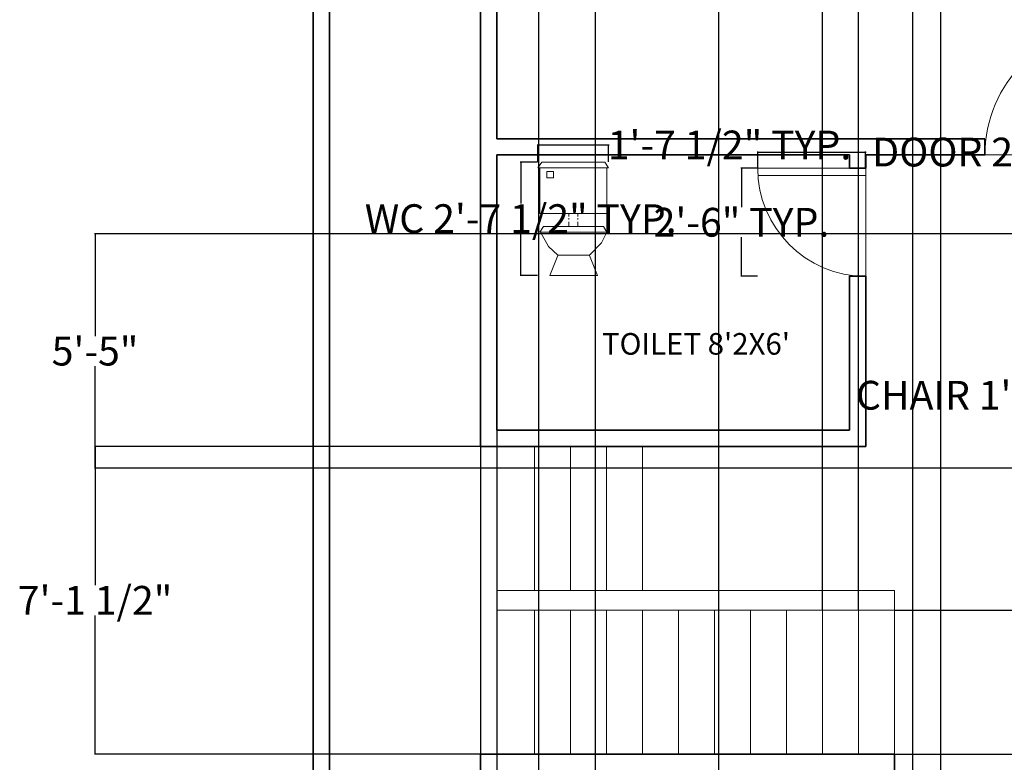
# Model space of a CAD drawing. Units: inches. Extents: x -438 to 102, y -60 to 1091.
# Tile 4 of 20: x -436 to -162, y 492 to 699. Entities that reach past the tile are written whole.
import ezdxf

# ---------------------------------------------------------------- set-up
doc = ezdxf.new("R2010")
doc.units = ezdxf.units.IN
doc.header["$MEASUREMENT"] = 0
for name, color, linetype, lineweight, true_color in [('A-ANNO-DIMS', 217, 'Continuous', 18, 0x93278f), ('A-DOOR', 30, 'Continuous', 18, 0xf26722), ('A-WALL', 2, 'Continuous', 35, 0xf1eb1f), ('C-PROP', 2, 'Continuous', 35, 0xf1eb1f)]:
    doc.layers.add(name, color=color, linetype=linetype, lineweight=lineweight, true_color=true_color)
for name, color, linetype, lineweight in [('A-AREA-IDEN', 4, 'Continuous', 18), ('A-FLOR-FIXT', 9, 'Continuous', 15), ('A-FLOR-STRS', 7, 'Continuous', 18)]:
    doc.layers.add(name, color=color, linetype=linetype, lineweight=lineweight)
doc.styles.get("Standard").update_dxf_attribs({"font": 'arial.ttf'})
doc.dimstyles.get("Standard").update_dxf_attribs({"dimtxt": 8, "dimasz": 0.18, "dimexe": 0.18, "dimexo": 0.0625, "dimgap": 0.09, "dimtad": 0, "dimtih": 1, "dimtoh": 1, "dimdec": 4, "dimzin": 0, "dimdsep": 46, "dimlunit": 3, "dimtxsty": 'Standard', "dimcen": 0.09, "dimadec": 0, "dimazin": 0, "dimtfac": 1, "dimtdec": 4, "dimtofl": 0, "dimtmove": 0, "dimatfit": 3, "dimfxl": 1, "dimtolj": 1, "dimtzin": 0, "dimarcsym": 0})

# ---------------------------------------------------------------- blocks, each defined once
blk = doc.blocks.new('WC-CLOSE-COUPLED')
for p, q in [((-9.84, -1.66, -13.5), (-8.74, 0, -13.5)), ((-8.74, 0, -13.5), (8.78, 0, -13.5)), ((9.84, -1.66, -13.5), (8.78, 0, -13.5)), ((-9.84, -1.66, -13.5), (9.84, -1.66, -13.5)), ((-9.27, -1.66, -13.5), (-9.27, -14.26, -13.5)), ((-7.35, -2.62, -13.5), (-7.35, -4.39, -13.5)), ((-5.45, -2.62, -13.5), (-7.35, -2.62, -13.5)), ((-5.45, -4.39, -13.5), (-5.45, -2.62, -13.5)), ((9.31, -14.26, -13.5), (9.31, -1.66, -13.5)), ((-7.35, -4.39, -13.5), (-5.45, -4.39, -13.5)), ((-9.27, -14.26, -13.5), (9.31, -14.26, -13.5)), ((-1.22, -15.15, -13.5), (-1.22, -14.23, -13.5)), ((-1.22, -15.97, -13.5), (-1.22, -15.56, -13.5)), ((0.02, -14.26, -13.5), (1.26, -14.26, -13.5)), ((1.26, -14.26, -13.5), (1.26, -15.15, -13.5)), ((1.26, -15.56, -13.5), (1.26, -15.97, -13.5)), ((-9.27, -19.49, -13.5), (-8.25, -17.89, -13.5)), ((-8.25, -17.89, -13.5), (8.4, -17.89, -13.5)), ((-1.22, -17.96, -13.5), (-1.22, -16.65, -13.5)), ((1.26, -17.96, -13.5), (-1.22, -17.96, -13.5)), ((1.26, -16.65, -13.5), (1.26, -17.96, -13.5)), ((9.31, -19.49, -13.5), (8.4, -17.89, -13.5)), ((-9.27, -19.49, -13.5), (9.31, -19.49, -13.5)), ((9.52, -19.49, -13.5), (-9.07, -19.49, -13.5)), ((-9.07, -19.49, -13.5), (-6.87, -23.48, -13.5)), ((7.85, -22.5, -13.5), (9.31, -19.49, -13.5)), ((-6.87, -23.48, -13.5), (-4.26, -25.89, -13.5)), ((4.51, -25.89, -13.5), (7.85, -22.5, -13.5)), ((-6.51, -31.49, -13.5), (-4.3, -25.95, -13.5)), ((-4.26, -25.89, -13.5), (4.51, -25.89, -13.5)), ((4.51, -25.89, -13.5), (-4.26, -25.89, -13.5)), ((6.76, -31.49, -13.5), (4.55, -25.95, -13.5)), ((-6.51, -31.49, -13.5), (6.76, -31.49, -13.5)), ((0.12, -31.49, -13.5), (-6.51, -31.49, -13.5))]:
    blk.add_line(p, q)
blk = doc.blocks.new('DOOR-SWING-36')
for p, q in [((-36, 0), (0, 0)), ((-2, 0), (-2, -36)), ((0, 0), (0, -36))]:
    blk.add_line(p, q)
blk.add_arc((0, 0), 36, 180, 270)
blk = doc.blocks.new('DOOR-SWING-30')
for p, q in [((0, 0), (-30, 0)), ((0, -30), (0, 0)), ((0, -2), (-30, -2))]:
    blk.add_line(p, q)
blk.add_arc((0, 0), 30, 180, 270)
blk = doc.blocks.new('*D14')
at = {"layer": 'A-ANNO-DIMS', "color": 0, "lineweight": -2, "transparency": 16777216}
for p, q in [((-99.6, 597.28), (-99.6, 594.06)), ((-78.92, 597.28), (-78.92, 594.06)), ((-99.6, 594.24), (-99.78, 594.24)), ((-79.1, 594.24), (-99.42, 594.24))]:
    blk.add_line(p, q, dxfattribs=at)
at = {"layer": 'A-ANNO-DIMS', "color": 0, "transparency": 16777216}
for points in [[(-99.42, 594.27), (-99.42, 594.21), (-99.6, 594.24)], [(-79.1, 594.27), (-79.1, 594.21), (-78.92, 594.24)]]:
    blk.add_solid(points, dxfattribs=at)
at = {"layer": 'Defpoints', "color": 0, "transparency": 16777216}
for p in [(-99.6, 597.34), (-78.92, 597.34), (-99.6, 594.24)]:
    blk.add_point(p, dxfattribs=at)
at = {"layer": 'A-ANNO-DIMS', "color": 0, "transparency": 16777216, "insert": (-152.46, 594.24), "char_height": 8, "attachment_point": 5}
blk.add_mtext('\\A1;CHAIR 1\'-8 1/2" TYP.', dxfattribs=at)
blk = doc.blocks.new('*D18')
at = {"layer": 'A-ANNO-DIMS', "color": 0, "lineweight": -2, "transparency": 16777216}
for p, q in [((-291.82, 659.04), (-296.67, 659.04)), ((-296.49, 658.86), (-296.49, 647.52)), ((-296.49, 627.73), (-296.49, 639.07)), ((-291.82, 627.55), (-296.67, 627.55))]:
    blk.add_line(p, q, dxfattribs=at)
at = {"layer": 'A-ANNO-DIMS', "color": 0, "transparency": 16777216}
for points in [[(-296.52, 658.86), (-296.46, 658.86), (-296.49, 659.04)], [(-296.52, 627.73), (-296.46, 627.73), (-296.49, 627.55)]]:
    blk.add_solid(points, dxfattribs=at)
at = {"layer": 'Defpoints', "color": 0, "transparency": 16777216}
for p in [(-296.49, 659.04), (-291.76, 659.04), (-291.76, 627.55)]:
    blk.add_point(p, dxfattribs=at)
at = {"layer": 'A-ANNO-DIMS', "color": 0, "transparency": 16777216, "insert": (-296.49, 643.3), "char_height": 8, "attachment_point": 5}
blk.add_mtext('\\A1;WC 2\'-7 1/2" TYP.', dxfattribs=at)
blk = doc.blocks.new('*D19')
at = {"layer": 'A-ANNO-DIMS', "color": 0, "lineweight": -2, "transparency": 16777216}
for p, q in [((-291.76, 659.11), (-291.76, 663.95)), ((-291.58, 663.77), (-272.26, 663.77)), ((-272.08, 659.11), (-272.08, 663.95)), ((-272.08, 663.77), (-271.9, 663.77))]:
    blk.add_line(p, q, dxfattribs=at)
at = {"layer": 'A-ANNO-DIMS', "color": 0, "transparency": 16777216}
for points in [[(-291.58, 663.8), (-291.58, 663.74), (-291.76, 663.77)], [(-272.26, 663.8), (-272.26, 663.74), (-272.08, 663.77)]]:
    blk.add_solid(points, dxfattribs=at)
at = {"layer": 'Defpoints', "color": 0, "transparency": 16777216}
for p in [(-272.08, 663.77), (-291.76, 659.04), (-272.08, 659.04)]:
    blk.add_point(p, dxfattribs=at)
at = {"layer": 'A-ANNO-DIMS', "color": 0, "transparency": 16777216, "insert": (-238.48, 663.77), "char_height": 8, "attachment_point": 5}
blk.add_mtext('\\A1;1\'-7 1/2" TYP.', dxfattribs=at)
blk = doc.blocks.new('*D22')
at = {"layer": 'A-ANNO-DIMS', "color": 0, "lineweight": -2, "transparency": 16777216}
for p, q in [((-230.65, 657.36), (-230.65, 661.98)), ((-230.47, 661.8), (-200.83, 661.8)), ((-200.65, 657.36), (-200.65, 661.98)), ((-200.65, 661.8), (-200.47, 661.8))]:
    blk.add_line(p, q, dxfattribs=at)
at = {"layer": 'A-ANNO-DIMS', "color": 0, "transparency": 16777216}
for points in [[(-230.47, 661.83), (-230.47, 661.77), (-230.65, 661.8)], [(-200.83, 661.83), (-200.83, 661.77), (-200.65, 661.8)]]:
    blk.add_solid(points, dxfattribs=at)
at = {"layer": 'Defpoints', "color": 0, "transparency": 16777216}
for p in [(-200.65, 661.8), (-230.65, 657.3), (-200.65, 657.3)]:
    blk.add_point(p, dxfattribs=at)
at = {"layer": 'A-ANNO-DIMS', "color": 0, "transparency": 16777216, "insert": (-157.88, 661.8), "char_height": 8, "attachment_point": 5}
blk.add_mtext('\\A1;DOOR 2\'-6" TYP.', dxfattribs=at)
blk = doc.blocks.new('*D23')
at = {"layer": 'A-ANNO-DIMS', "color": 0, "lineweight": -2, "transparency": 16777216}
for p, q in [((-230.71, 657.3), (-235.33, 657.3)), ((-235.15, 657.12), (-235.15, 646.47)), ((-235.15, 627.48), (-235.15, 638.13)), ((-230.71, 627.3), (-235.33, 627.3))]:
    blk.add_line(p, q, dxfattribs=at)
at = {"layer": 'A-ANNO-DIMS', "color": 0, "transparency": 16777216}
for points in [[(-235.18, 657.12), (-235.12, 657.12), (-235.15, 657.3)], [(-235.18, 627.48), (-235.12, 627.48), (-235.15, 627.3)]]:
    blk.add_solid(points, dxfattribs=at)
at = {"layer": 'Defpoints', "color": 0, "transparency": 16777216}
for p in [(-235.15, 657.3), (-230.65, 657.3), (-230.65, 627.3)]:
    blk.add_point(p, dxfattribs=at)
at = {"layer": 'A-ANNO-DIMS', "color": 0, "transparency": 16777216, "insert": (-235.15, 642.3), "char_height": 8, "attachment_point": 5}
blk.add_mtext('\\A1;2\'-6" TYP.', dxfattribs=at)
blk = doc.blocks.new('*D29')
at = {"layer": 'A-ANNO-DIMS', "color": 0, "lineweight": -2, "transparency": 16777216}
for p, q in [((-303.15, 494.44), (-303.15, -48.58)), ((-192.65, 494.44), (-192.65, -48.58)), ((-302.97, -48.4), (-267.94, -48.4)), ((-192.83, -48.4), (-227.85, -48.4))]:
    blk.add_line(p, q, dxfattribs=at)
at = {"layer": 'A-ANNO-DIMS', "color": 0, "transparency": 16777216}
for points in [[(-302.97, -48.37), (-302.97, -48.43), (-303.15, -48.4)], [(-192.83, -48.37), (-192.83, -48.43), (-192.65, -48.4)]]:
    blk.add_solid(points, dxfattribs=at)
at = {"layer": 'Defpoints', "color": 0, "transparency": 16777216}
for p in [(-303.15, 494.5), (-192.65, 494.5), (-192.65, -48.4)]:
    blk.add_point(p, dxfattribs=at)
at = {"layer": 'A-ANNO-DIMS', "color": 0, "transparency": 16777216, "insert": (-247.9, -48.4), "char_height": 8, "attachment_point": 5}
blk.add_mtext('\\A1;9\'-2 1/2"', dxfattribs=at)
blk = doc.blocks.new('*D30')
at = {"layer": 'A-ANNO-DIMS', "color": 0, "lineweight": -2, "transparency": 16777216}
for p, q in [((-303.21, 580), (-414.94, 580)), ((-414.76, 579.82), (-414.76, 541.48)), ((-414.76, 494.68), (-414.76, 533.02)), ((-303.21, 494.5), (-414.94, 494.5))]:
    blk.add_line(p, q, dxfattribs=at)
at = {"layer": 'A-ANNO-DIMS', "color": 0, "transparency": 16777216}
for points in [[(-414.79, 579.82), (-414.73, 579.82), (-414.76, 580)], [(-414.79, 494.68), (-414.73, 494.68), (-414.76, 494.5)]]:
    blk.add_solid(points, dxfattribs=at)
at = {"layer": 'Defpoints', "color": 0, "transparency": 16777216}
for p in [(-414.76, 580), (-303.15, 580), (-303.15, 494.5)]:
    blk.add_point(p, dxfattribs=at)
at = {"layer": 'A-ANNO-DIMS', "color": 0, "transparency": 16777216, "insert": (-414.76, 537.25), "char_height": 8, "attachment_point": 5}
blk.add_mtext('\\A1;7\'-1 1/2"', dxfattribs=at)
blk = doc.blocks.new('*D32')
at = {"layer": 'A-ANNO-DIMS', "color": 0, "lineweight": -2, "transparency": 16777216}
for p, q in [((-303.15, 584.44), (-303.15, -48.58)), ((-307.65, 579.94), (-307.65, -48.58)), ((-307.47, -48.4), (-303.33, -48.4)), ((-303.15, -48.4), (-302.97, -48.4))]:
    blk.add_line(p, q, dxfattribs=at)
at = {"layer": 'A-ANNO-DIMS', "color": 0, "transparency": 16777216}
for points in [[(-307.47, -48.37), (-307.47, -48.43), (-307.65, -48.4)], [(-303.33, -48.37), (-303.33, -48.43), (-303.15, -48.4)]]:
    blk.add_solid(points, dxfattribs=at)
at = {"layer": 'Defpoints', "color": 0, "transparency": 16777216}
for p in [(-303.15, 584.5), (-307.65, 580), (-303.15, -48.4)]:
    blk.add_point(p, dxfattribs=at)
at = {"layer": 'A-ANNO-DIMS', "color": 0, "transparency": 16777216, "insert": (-282.92, -48.4), "char_height": 8, "attachment_point": 5}
blk.add_mtext('\\A1;0\'-4 1/2"', dxfattribs=at)
blk = doc.blocks.new('*D37')
at = {"layer": 'A-ANNO-DIMS', "color": 0, "lineweight": -2, "transparency": 16777216}
for p, q in [((-179.8, 234.94), (-179.8, 1079.58)), ((-179.62, 1079.4), (-176.98, 1079.4)), ((-134.26, 1079.4), (-136.9, 1079.4)), ((-134.08, 234.94), (-134.08, 1079.58))]:
    blk.add_line(p, q, dxfattribs=at)
at = {"layer": 'A-ANNO-DIMS', "color": 0, "transparency": 16777216}
for points in [[(-179.62, 1079.43), (-179.62, 1079.37), (-179.8, 1079.4)], [(-134.26, 1079.43), (-134.26, 1079.37), (-134.08, 1079.4)]]:
    blk.add_solid(points, dxfattribs=at)
at = {"layer": 'Defpoints', "color": 0, "transparency": 16777216}
for p in [(-134.08, 1079.4), (-179.8, 234.88), (-134.08, 234.88)]:
    blk.add_point(p, dxfattribs=at)
at = {"layer": 'A-ANNO-DIMS', "color": 0, "transparency": 16777216, "insert": (-156.94, 1079.4), "char_height": 8, "attachment_point": 5}
blk.add_mtext('\\A1;3\'-9 1/2"', dxfattribs=at)
blk = doc.blocks.new('*D46')
at = {"layer": 'A-ANNO-DIMS', "color": 0, "lineweight": -2, "transparency": 16777216}
for p, q in [((-72.95, 639.04), (-414.94, 639.04)), ((-414.76, 638.86), (-414.76, 610.65)), ((-414.76, 574.12), (-414.76, 602.33)), ((-73.11, 573.94), (-414.94, 573.94))]:
    blk.add_line(p, q, dxfattribs=at)
at = {"layer": 'A-ANNO-DIMS', "color": 0, "transparency": 16777216}
for points in [[(-414.79, 638.86), (-414.73, 638.86), (-414.76, 639.04)], [(-414.79, 574.12), (-414.73, 574.12), (-414.76, 573.94)]]:
    blk.add_solid(points, dxfattribs=at)
at = {"layer": 'Defpoints', "color": 0, "transparency": 16777216}
for p in [(-414.76, 639.04), (-72.89, 639.04), (-73.05, 573.94)]:
    blk.add_point(p, dxfattribs=at)
at = {"layer": 'A-ANNO-DIMS', "color": 0, "transparency": 16777216, "insert": (-414.76, 606.49), "char_height": 8, "attachment_point": 5}
blk.add_mtext('\\A1;5\'-5"', dxfattribs=at)
blk = doc.blocks.new('*D51')
at = {"layer": 'A-ANNO-DIMS', "color": 0, "lineweight": -2, "transparency": 16777216}
for p, q in [((-291.54, 847), (-291.54, -48.58)), ((-275.79, 847), (-275.79, -48.58)), ((-291.36, -48.4), (-275.97, -48.4)), ((-275.79, -48.4), (-275.61, -48.4))]:
    blk.add_line(p, q, dxfattribs=at)
at = {"layer": 'A-ANNO-DIMS', "color": 0, "transparency": 16777216}
for points in [[(-291.36, -48.37), (-291.36, -48.43), (-291.54, -48.4)], [(-275.97, -48.37), (-275.97, -48.43), (-275.79, -48.4)]]:
    blk.add_solid(points, dxfattribs=at)
at = {"layer": 'Defpoints', "color": 0, "transparency": 16777216}
for p in [(-291.54, 847.06), (-275.79, 847.06), (-275.79, -48.4)]:
    blk.add_point(p, dxfattribs=at)
at = {"layer": 'A-ANNO-DIMS', "color": 0, "transparency": 16777216, "insert": (-255.95, -48.4), "char_height": 8, "attachment_point": 5}
blk.add_mtext('\\A1;1\'-3 1/2"', dxfattribs=at)
blk = doc.blocks.new('*D55')
at = {"layer": 'A-ANNO-DIMS', "color": 0, "lineweight": -2, "transparency": 16777216}
for p, q in [((-241.57, 808.32), (-241.57, -48.58)), ((-187.65, 801.94), (-187.65, -48.58)), ((-241.39, -48.4), (-225.49, -48.4)), ((-187.83, -48.4), (-203.72, -48.4))]:
    blk.add_line(p, q, dxfattribs=at)
at = {"layer": 'A-ANNO-DIMS', "color": 0, "transparency": 16777216}
for points in [[(-241.39, -48.37), (-241.39, -48.43), (-241.57, -48.4)], [(-187.83, -48.37), (-187.83, -48.43), (-187.65, -48.4)]]:
    blk.add_solid(points, dxfattribs=at)
at = {"layer": 'Defpoints', "color": 0, "transparency": 16777216}
for p in [(-241.57, 808.38), (-187.65, 802), (-187.65, -48.4)]:
    blk.add_point(p, dxfattribs=at)
at = {"layer": 'A-ANNO-DIMS', "color": 0, "transparency": 16777216, "insert": (-214.61, -48.4), "char_height": 8, "attachment_point": 5}
blk.add_mtext('\\A1;4\'-6"', dxfattribs=at)
blk = doc.blocks.new('*D60')
at = {"layer": 'A-ANNO-DIMS', "color": 0, "lineweight": -2, "transparency": 16777216}
for p, q in [((-192.58, 534.5), (81.43, 534.5)), ((81.25, 534.32), (81.25, 518.68)), ((81.25, 494.68), (81.25, 510.32)), ((-192.58, 494.5), (81.43, 494.5))]:
    blk.add_line(p, q, dxfattribs=at)
at = {"layer": 'A-ANNO-DIMS', "color": 0, "transparency": 16777216}
for points in [[(81.22, 534.32), (81.28, 534.32), (81.25, 534.5)], [(81.22, 494.68), (81.28, 494.68), (81.25, 494.5)]]:
    blk.add_solid(points, dxfattribs=at)
at = {"layer": 'Defpoints', "color": 0, "transparency": 16777216}
for p in [(-192.65, 534.5), (81.25, 534.5), (-192.65, 494.5)]:
    blk.add_point(p, dxfattribs=at)
at = {"layer": 'A-ANNO-DIMS', "color": 0, "transparency": 16777216, "insert": (81.25, 514.5), "char_height": 8, "attachment_point": 5}
blk.add_mtext('\\A1;3\'-4"', dxfattribs=at)
blk = doc.blocks.new('*D61')
at = {"layer": 'A-ANNO-DIMS', "color": 0, "lineweight": -2, "transparency": 16777216}
for p, q in [((-212.65, 1079.4), (-212.83, 1079.4)), ((-212.65, 534.56), (-212.65, 1079.58)), ((-202.83, 1079.4), (-212.47, 1079.4)), ((-202.65, 534.56), (-202.65, 1079.58))]:
    blk.add_line(p, q, dxfattribs=at)
at = {"layer": 'A-ANNO-DIMS', "color": 0, "transparency": 16777216}
for points in [[(-212.47, 1079.43), (-212.47, 1079.37), (-212.65, 1079.4)], [(-202.83, 1079.43), (-202.83, 1079.37), (-202.65, 1079.4)]]:
    blk.add_solid(points, dxfattribs=at)
at = {"layer": 'Defpoints', "color": 0, "transparency": 16777216}
for p in [(-212.65, 1079.4), (-212.65, 534.5), (-202.65, 534.5)]:
    blk.add_point(p, dxfattribs=at)
at = {"layer": 'A-ANNO-DIMS', "color": 0, "transparency": 16777216, "insert": (-226.66, 1079.4), "char_height": 8, "attachment_point": 5}
blk.add_mtext('\\A1;0\'-10"', dxfattribs=at)

msp = doc.modelspace()

# ---------------------------------------------------------------- linework, layer by layer
at = {"layer": 'A-FLOR-STRS'}
for p, q in [((-303.14649, 579.99939), (-303.14649, 494.49939)), ((-292.64649, 539.99939), (-292.64649, 579.99939)), ((-282.64649, 539.99939), (-282.64649, 579.99939)), ((-272.64649, 539.99939), (-272.64649, 579.99939)), ((-262.64649, 539.99939), (-262.64649, 579.99939)), ((-192.64649, 539.99939), (-303.14649, 539.99939)), ((-192.64649, 534.49939), (-192.64649, 539.99939)), ((-192.64649, 534.49939), (-303.14649, 534.49939)), ((-292.64649, 494.49939), (-292.64649, 534.49939)), ((-282.64649, 494.49939), (-282.64649, 534.49939)), ((-272.64649, 494.49939), (-272.64649, 534.49939)), ((-262.64649, 494.49939), (-262.64649, 534.49939)), ((-252.64649, 494.49939), (-252.64649, 534.49939)), ((-242.64649, 494.49939), (-242.64649, 534.49939)), ((-232.64649, 494.49939), (-232.64649, 534.49939)), ((-222.64649, 494.49939), (-222.64649, 534.49939)), ((-212.64649, 494.49939), (-212.64649, 534.49939)), ((-202.64649, 494.49939), (-202.64649, 534.49939)), ((-192.64649, 494.49939), (-192.64649, 534.49939))]:
    msp.add_line(p, q, dxfattribs=at)
at = {"layer": 'A-WALL'}
for p, q in [((-307.64649, 897.99939), (-307.64649, 579.99939)), ((-303.14649, 797.49939), (-303.14649, 665.49939)), ((-167.50148, 665.49939), (-303.14649, 665.49939)), ((-167.50148, 665.49939), (-167.50148, 660.99939)), ((-303.14649, 660.99939), (-303.14649, 584.49939)), ((-205.14649, 660.99939), (-303.14649, 660.99939)), ((-205.14649, 660.99939), (-205.14649, 657.30022)), ((-200.64649, 660.99939), (-200.64649, 657.30022)), ((-167.50148, 660.99939), (-200.64649, 660.99939)), ((-200.64649, 657.30022), (-205.14649, 657.30022)), ((-205.14649, 627.30022), (-205.14649, 584.49939)), ((-200.64649, 627.30022), (-205.14649, 627.30022)), ((-200.64649, 627.30022), (-200.64649, 579.99939)), ((-205.14649, 584.49939), (-303.14649, 584.49939)), ((-200.64649, 579.99939), (-307.64649, 579.99939)), ((-192.64649, 494.49939), (-307.64649, 494.49939)), ((-307.64649, 494.49939), (-307.64649, 489.99939)), ((-192.64649, 494.49939), (-192.64649, 484.46947))]:
    msp.add_line(p, q, dxfattribs=at)
at = {"layer": 'C-PROP'}
for p, q in [((-354.14649, 1026.99939), (-354.14649, 3.99939)), ((-349.64649, 897.99939), (-349.64649, 8.49939))]:
    msp.add_line(p, q, dxfattribs=at)

# ---------------------------------------------------------------- block references
at = {"layer": 'A-DOOR', "extrusion": (0, 0, -1), "zscale": -1, "rotation": 180}
msp.add_blockref('DOOR-SWING-36', (131.50148, 660.99939), dxfattribs=at)
at = {"layer": 'A-DOOR'}
msp.add_blockref('DOOR-SWING-30', (-200.64649, 657.30022), dxfattribs=at)
at = {"layer": 'A-FLOR-FIXT'}
msp.add_blockref('WC-CLOSE-COUPLED', (-281.92, 659.04), dxfattribs=at)

# ---------------------------------------------------------------- texts
at = {"layer": 'A-AREA-IDEN'}
msp.add_text("TOILET 8'2X6'", height=6, dxfattribs=at).set_placement((-273.92034, 605.51399))

# ---------------------------------------------------------------- dimensions: what is measured, and where the dimension line sits
at = {"layer": 'A-ANNO-DIMS'}
for base, p1, p2, picture, middle in [((-134.07948, 1079.39939), (-179.79585, 234.87846), (-134.07948, 234.87846), '*D37', (-156.93767, 1079.39939)), ((-212.64649, 1079.39939), (-202.64649, 534.49939), (-212.64649, 534.49939), '*D61', (-226.65728, 1079.39939)), ((-275.79225, -48.40061), (-291.54025, 847.06395), (-275.79225, 847.06395), '*D51', (-255.94517, -48.40061)), ((-187.64649, -48.40061), (-241.57044, 808.38394), (-187.64649, 801.99939), '*D55', (-214.60846, -48.40061)), ((-303.14649, -48.40061), (-307.64649, 579.99939), (-303.14649, 584.49939), '*D32', (-282.92287, -48.40061)), ((-192.64649, -48.40061), (-303.14649, 494.49939), (-192.64649, 494.49939), '*D29', (-247.89649, -48.40061))]:
    dim = msp.add_linear_dim(base=base, p1=p1, p2=p2, dimstyle='Standard', override={"dimdec": 1, "dimlfac": 1, "dimrnd": 0, "dimzin": 1, "dimdsep": 46, "dimlunit": 4, "dimfrac": 2}, dxfattribs=at)
    dim.commit()
    dim.dimension.update_dxf_attribs({"geometry": picture, "text_midpoint": middle})
for base, p1, p2, text, picture, middle in [((-272.07633, 663.76783), (-291.76133, 659.04343), (-272.07633, 659.04343), '<> TYP.', '*D19', (-238.48028, 663.76783)), ((-200.64649, 661.80022), (-230.64649, 657.30022), (-200.64649, 657.30022), 'DOOR <> TYP.', '*D22', (-157.87717, 661.80022))]:
    dim = msp.add_linear_dim(base=base, p1=p1, p2=p2, text=text, dimstyle='Standard', override={"dimdec": 1, "dimlfac": 1, "dimrnd": 0, "dimzin": 1, "dimdsep": 46, "dimlunit": 4, "dimfrac": 2}, dxfattribs=at)
    dim.commit()
    dim.dimension.update_dxf_attribs({"geometry": picture, "text_midpoint": middle})
for base, p1, p2, angle, text, picture, middle in [((-296.48573, 659.04343), (-291.76133, 627.54743), (-291.76133, 659.04343), 90, 'WC <> TYP.', '*D18', (-296.48573, 643.29543)), ((-235.14649, 657.30022), (-230.64649, 627.30022), (-230.64649, 657.30022), 90, '<> TYP.', '*D23', (-235.14649, 642.30022)), ((-99.59998, 594.23876), (-78.919, 597.34091), (-99.59998, 597.34091), 180, 'CHAIR <> TYP.', '*D14', (-152.4648, 594.23876))]:
    dim = msp.add_linear_dim(base=base, p1=p1, p2=p2, angle=angle, text=text, dimstyle='Standard', override={"dimdec": 1, "dimlfac": 1, "dimrnd": 0, "dimzin": 1, "dimdsep": 46, "dimlunit": 4, "dimfrac": 2}, dxfattribs=at)
    dim.commit()
    dim.dimension.update_dxf_attribs({"geometry": picture, "text_midpoint": middle})
for base, p1, p2, picture, middle in [((-414.76009, 639.04071), (-73.0511, 573.94064), (-72.889, 639.04071), '*D46', (-414.76009, 606.49067)), ((-414.76009, 579.99939), (-303.14649, 494.49939), (-303.14649, 579.99939), '*D30', (-414.76009, 537.24939)), ((81.25351, 534.49939), (-192.64649, 494.49939), (-192.64649, 534.49939), '*D60', (81.25351, 514.49939))]:
    dim = msp.add_linear_dim(base=base, p1=p1, p2=p2, angle=90, dimstyle='Standard', override={"dimdec": 1, "dimlfac": 1, "dimrnd": 0, "dimzin": 1, "dimdsep": 46, "dimlunit": 4, "dimfrac": 2}, dxfattribs=at)
    dim.commit()
    dim.dimension.update_dxf_attribs({"geometry": picture, "text_midpoint": middle})

doc.saveas('drawing.dxf')
